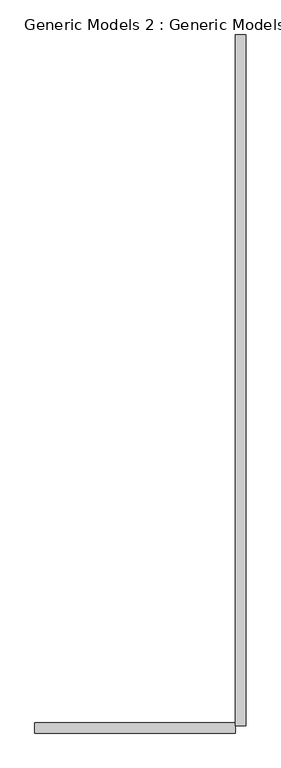
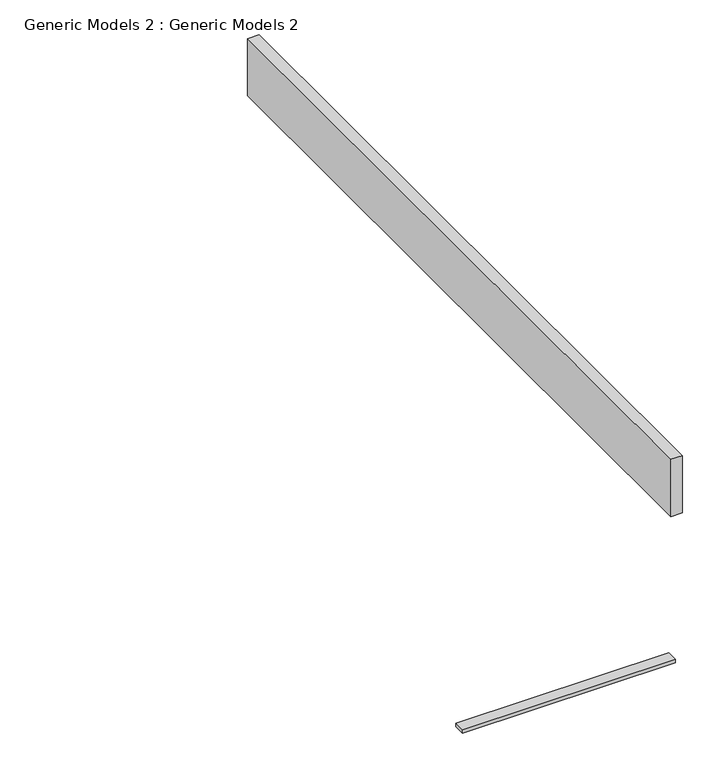
"""IFC4 building model written with IfcOpenShell, lengths in millimetres: proxy geometry, Generic Models 2 : Generic Models 2."""

from ifc_helpers import new_model, si_unit, frame, origin, place, context, project, spatial, polyline, outline, extrude, source, transform, mapped, element, save


def generic_models_2_generic_models_2_9dd516d1(model_context):
    return source(origin(), model_context, "Body", "SweptSolid", [
        extrude(outline(polyline([(-10720.4161422, 5487.8132242), (-10720.4161422, -9466.2958238), (-10949.0161422, -9466.2958238), (-10949.0161422, 5487.8132242), (-10720.4161422, 5487.8132242)])), frame((0.0, 0.0, 6400.8), z_axis=(0.0, 0.0, 1.0), x_axis=(1.0, 0.0, 0.0)), (0.0, 0.0, 1.0), 1234.8513671),
        extrude(outline(polyline([(-15292.4161422, -9625.1422165), (-15292.4161422, -9396.5867758), (-10949.0161422, -9396.5867758), (-10949.0161422, -9625.1422165), (-15292.4161422, -9625.1422165)])), frame((0.0, 0.0, 3352.8), z_axis=(0.0, 0.0, 1.0), x_axis=(1.0, 0.0, 0.0)), (0.0, 0.0, 1.0), 76.2),
    ])


if __name__ == "__main__":
    model = new_model("IFC4")
    model_context = context("Model", 3, world=origin())
    ifc_project = project(units=[si_unit("LENGTHUNIT", "METRE", prefix="MILLI")], contexts=[model_context])
    site = spatial("IfcSite", under=ifc_project)
    building = spatial("IfcBuilding", under=site)
    placement = place(None, origin())
    generic_models_2_generic_models_2_shape = generic_models_2_generic_models_2_9dd516d1(model_context)
    element("IfcBuildingElementProxy", 1, Name="Generic Models 2 : Generic Models 2", ObjectType="Generic Models 2 : Generic Models 2", at=placement, inside=building, context=model_context, shape_type="MappedRepresentation", body=[
        mapped(generic_models_2_generic_models_2_shape, transform((0.0, 0.0, 0.0), x_axis=(1.0, 0.0, 0.0), y_axis=(0.0, 1.0, 0.0), z_axis=(0.0, 0.0, 1.0))),
    ])
    save(model, "model.ifc")
